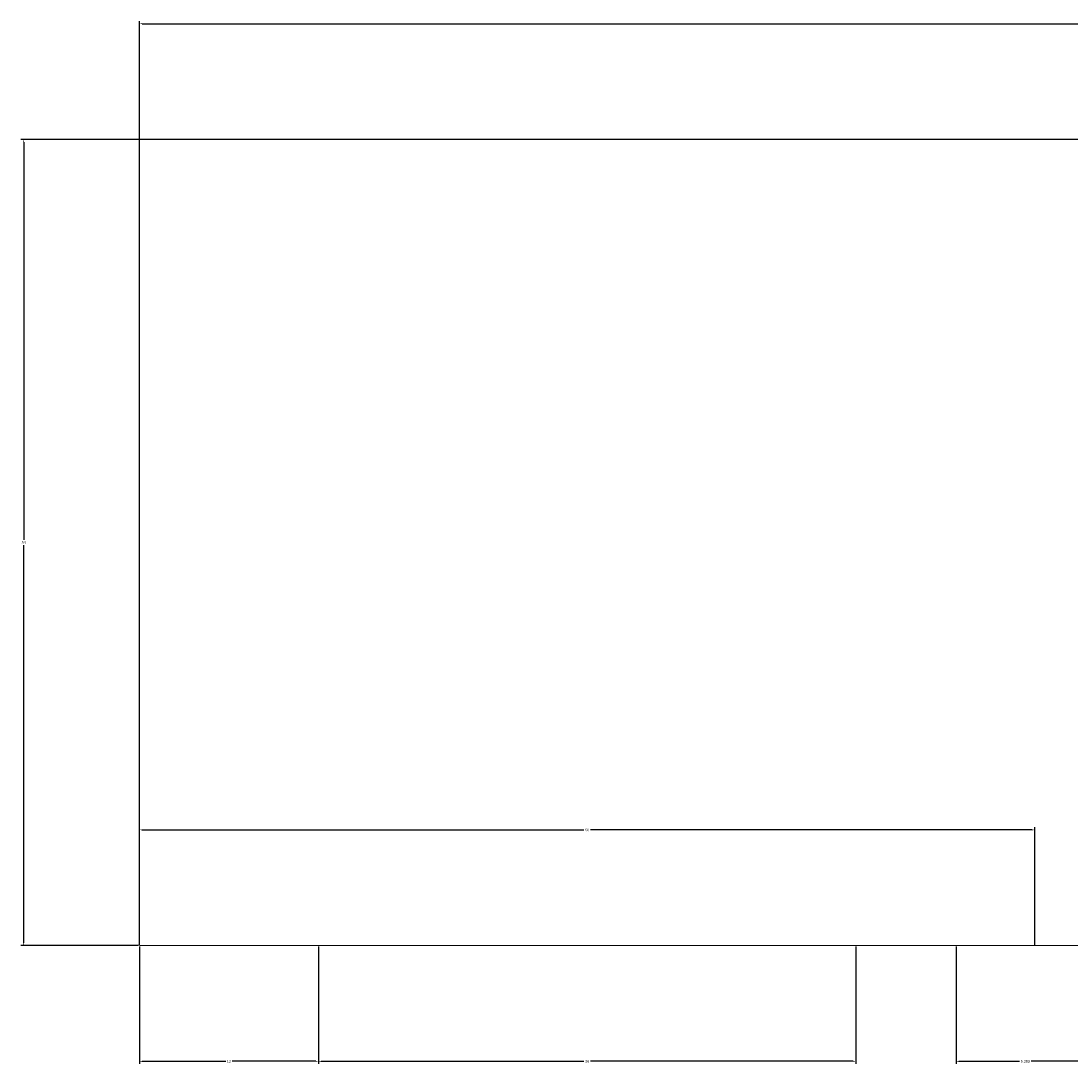
# Model space of a CAD drawing. Units: millimetres. Extents: x 223 to 381, y -8 to 62.
# Tile 1 of 5: x 223 to 293, y -8 to 62. Entities that reach past the tile are written whole.
import ezdxf

# ---------------------------------------------------------------- set-up
doc = ezdxf.new("R2010")
doc.units = ezdxf.units.MM
doc.layers.add('M-CONS', color=8, linetype='Continuous', lineweight=13)
doc.layers.add('M-DIMS', color=2, linetype='Continuous', lineweight=18)
doc.styles.get("Standard").update_dxf_attribs({"font": 'arial.ttf'})
doc.dimstyles.get("Standard").update_dxf_attribs({"dimtxt": 0.18, "dimasz": 0.18, "dimexe": 0.18, "dimexo": 0.0625, "dimgap": 0.09, "dimtad": 0, "dimtih": 1, "dimtoh": 1, "dimdec": 4, "dimzin": 0, "dimdsep": 46, "dimtxsty": 'Standard', "dimcen": 0.09, "dimadec": 0, "dimazin": 0, "dimtfac": 1, "dimtdec": 4, "dimtofl": 0, "dimtmove": 0, "dimatfit": 3, "dimfxl": 1, "dimtolj": 1, "dimtzin": 0, "dimarcsym": 0})

# ---------------------------------------------------------------- blocks, each defined once
blk = doc.blocks.new('*D1')
at = {"layer": 'Defpoints', "color": 0, "transparency": 16777216}
for p in [(372.659, 61.75), (372.659, 27), (230.659, 0)]:
    blk.add_point(p, dxfattribs=at)
at = {"layer": 'M-DIMS', "color": 0, "lineweight": -2, "transparency": 16777216}
for p, q in [((230.659, 0.062), (230.659, 61.93)), ((372.659, 27.062), (372.659, 61.93)), ((230.839, 61.75), (301.38, 61.75)), ((372.479, 61.75), (301.939, 61.75))]:
    blk.add_line(p, q, dxfattribs=at)
at = {"layer": 'M-DIMS', "color": 0, "transparency": 16777216}
for points in [[(230.839, 61.78), (230.839, 61.72), (230.659, 61.75)], [(372.479, 61.78), (372.479, 61.72), (372.659, 61.75)]]:
    blk.add_solid(points, dxfattribs=at)
at = {"layer": 'M-DIMS', "color": 0, "transparency": 16777216, "insert": (301.659, 61.75), "char_height": 0.18, "attachment_point": 5}
blk.add_mtext('\\A1;142', dxfattribs=at)
blk = doc.blocks.new('*D2')
at = {"layer": 'Defpoints', "color": 0, "transparency": 16777216}
for p in [(290.659, 7.75), (230.659, 0), (290.659, 0)]:
    blk.add_point(p, dxfattribs=at)
at = {"layer": 'M-DIMS', "color": 0, "lineweight": -2, "transparency": 16777216}
for p, q in [((230.659, 0.062), (230.659, 7.93)), ((230.839, 7.75), (260.44, 7.75)), ((290.479, 7.75), (260.878, 7.75)), ((290.659, 0.062), (290.659, 7.93))]:
    blk.add_line(p, q, dxfattribs=at)
at = {"layer": 'M-DIMS', "color": 0, "transparency": 16777216}
for points in [[(230.839, 7.78), (230.839, 7.72), (230.659, 7.75)], [(290.479, 7.78), (290.479, 7.72), (290.659, 7.75)]]:
    blk.add_solid(points, dxfattribs=at)
at = {"layer": 'M-DIMS', "color": 0, "transparency": 16777216, "insert": (260.659, 7.75), "char_height": 0.18, "attachment_point": 5}
blk.add_mtext('\\A1;60', dxfattribs=at)
blk = doc.blocks.new('*D3')
at = {"layer": 'Defpoints', "color": 0, "transparency": 16777216}
for p in [(230.659, 0), (242.659, 0), (242.659, -7.75)]:
    blk.add_point(p, dxfattribs=at)
at = {"layer": 'M-DIMS', "color": 0, "lineweight": -2, "transparency": 16777216}
for p, q in [((230.659, -0.062), (230.659, -7.93)), ((242.659, -0.062), (242.659, -7.93)), ((230.839, -7.75), (236.45, -7.75)), ((242.479, -7.75), (236.869, -7.75))]:
    blk.add_line(p, q, dxfattribs=at)
at = {"layer": 'M-DIMS', "color": 0, "transparency": 16777216}
for points in [[(230.839, -7.72), (230.839, -7.78), (230.659, -7.75)], [(242.479, -7.72), (242.479, -7.78), (242.659, -7.75)]]:
    blk.add_solid(points, dxfattribs=at)
at = {"layer": 'M-DIMS', "color": 0, "transparency": 16777216, "insert": (236.659, -7.75), "char_height": 0.18, "attachment_point": 5}
blk.add_mtext('\\A1;12', dxfattribs=at)
blk = doc.blocks.new('*D4')
at = {"layer": 'Defpoints', "color": 0, "transparency": 16777216}
for p in [(242.659, 0), (278.659, 0), (278.659, -7.75)]:
    blk.add_point(p, dxfattribs=at)
at = {"layer": 'M-DIMS', "color": 0, "lineweight": -2, "transparency": 16777216}
for p, q in [((242.659, -0.062), (242.659, -7.93)), ((278.659, -0.062), (278.659, -7.93)), ((242.839, -7.75), (260.44, -7.75)), ((278.479, -7.75), (260.878, -7.75))]:
    blk.add_line(p, q, dxfattribs=at)
at = {"layer": 'M-DIMS', "color": 0, "transparency": 16777216}
for points in [[(242.839, -7.72), (242.839, -7.78), (242.659, -7.75)], [(278.479, -7.72), (278.479, -7.78), (278.659, -7.75)]]:
    blk.add_solid(points, dxfattribs=at)
at = {"layer": 'M-DIMS', "color": 0, "transparency": 16777216, "insert": (260.659, -7.75), "char_height": 0.18, "attachment_point": 5}
blk.add_mtext('\\A1;36', dxfattribs=at)
blk = doc.blocks.new('*D5')
at = {"layer": 'Defpoints', "color": 0, "transparency": 16777216}
for p in [(285.376, 0), (294.659, 0), (294.659, -7.75)]:
    blk.add_point(p, dxfattribs=at)
at = {"layer": 'M-DIMS', "color": 0, "lineweight": -2, "transparency": 16777216}
for p, q in [((285.376, -0.062), (285.376, -7.93)), ((294.659, -0.062), (294.659, -7.93)), ((285.556, -7.75), (289.624, -7.75)), ((294.479, -7.75), (290.411, -7.75))]:
    blk.add_line(p, q, dxfattribs=at)
at = {"layer": 'M-DIMS', "color": 0, "transparency": 16777216}
for points in [[(285.556, -7.72), (285.556, -7.78), (285.376, -7.75)], [(294.479, -7.72), (294.479, -7.78), (294.659, -7.75)]]:
    blk.add_solid(points, dxfattribs=at)
at = {"layer": 'M-DIMS', "color": 0, "transparency": 16777216, "insert": (290.018, -7.75), "char_height": 0.18, "attachment_point": 5}
blk.add_mtext('\\A1;9.283', dxfattribs=at)
blk = doc.blocks.new('*D11')
at = {"layer": 'Defpoints', "color": 0, "transparency": 16777216}
for p in [(222.909, 54), (294.659, 54), (230.659, 0)]:
    blk.add_point(p, dxfattribs=at)
at = {"layer": 'M-DIMS', "color": 0, "lineweight": -2, "transparency": 16777216}
for p, q in [((294.597, 54), (222.729, 54)), ((222.909, 53.82), (222.909, 27.182)), ((222.909, 0.18), (222.909, 26.818)), ((230.597, 0), (222.729, 0))]:
    blk.add_line(p, q, dxfattribs=at)
at = {"layer": 'M-DIMS', "color": 0, "transparency": 16777216}
for points in [[(222.879, 53.82), (222.939, 53.82), (222.909, 54)], [(222.879, 0.18), (222.939, 0.18), (222.909, 0)]]:
    blk.add_solid(points, dxfattribs=at)
at = {"layer": 'M-DIMS', "color": 0, "transparency": 16777216, "insert": (222.909, 27), "char_height": 0.18, "attachment_point": 5}
blk.add_mtext('\\A1;54', dxfattribs=at)

msp = doc.modelspace()

# ---------------------------------------------------------------- linework, layer by layer
at = {"layer": 'M-CONS', "extrusion": (0, -1, 0)}
for p, q in [((260.6592, 0, 97.6363), (332.6592, 0, 97.6363)), ((294.6592, 0, 50.3189), (285.3762, 0, 50.6343))]:
    msp.add_line(p, q, dxfattribs=at)
for radius in [30, 18]:
    msp.add_circle((260.6592, 67.6363), radius, dxfattribs=at)

# ---------------------------------------------------------------- dimensions: what is measured, and where the dimension line sits
at = {"layer": 'M-DIMS'}
for base, p1, p2, override, picture, middle in [((372.6592, 61.75), (230.6592, 0), (372.6592, 27), {"dimdec": 0, "dimlfac": 1, "dimrnd": 0, "dimzin": 0, "dimdsep": 46, "dimlunit": 2}, '*D1', (301.6592, 61.75)), ((290.6592, 7.75), (230.6592, 0), (290.6592, 0), {"dimdec": 0, "dimlfac": 1, "dimrnd": 0, "dimzin": 0, "dimdsep": 46, "dimlunit": 2}, '*D2', (260.6592, 7.75)), ((242.6592, -7.75), (230.6592, 0), (242.6592, 0), {"dimdec": 0, "dimlfac": 1, "dimrnd": 0, "dimzin": 0, "dimdsep": 46, "dimlunit": 2}, '*D3', (236.6592, -7.75)), ((278.6592, -7.75), (242.6592, 0), (278.6592, 0), {"dimdec": 0, "dimlfac": 1, "dimrnd": 0, "dimzin": 0, "dimdsep": 46, "dimlunit": 2}, '*D4', (260.6592, -7.75)), ((294.6592, -7.75), (285.3762, 0), (294.6592, 0), {"dimdec": 3, "dimlfac": 1, "dimrnd": 0, "dimzin": 0, "dimdsep": 46, "dimlunit": 2}, '*D5', (290.0177, -7.75))]:
    dim = msp.add_linear_dim(base=base, p1=p1, p2=p2, dimstyle='Standard', override=override, dxfattribs=at)
    dim.commit()
    dim.dimension.update_dxf_attribs({"geometry": picture, "text_midpoint": middle})
dim = msp.add_linear_dim(base=(222.9092, 54), p1=(230.6592, 0), p2=(294.6592, 54), angle=90, dimstyle='Standard', override={"dimdec": 0, "dimlfac": 1, "dimrnd": 0, "dimzin": 0, "dimdsep": 46, "dimlunit": 2}, dxfattribs=at)
dim.commit()
dim.dimension.update_dxf_attribs({"geometry": '*D11', "text_midpoint": (222.9092, 27)})

doc.saveas('drawing.dxf')
